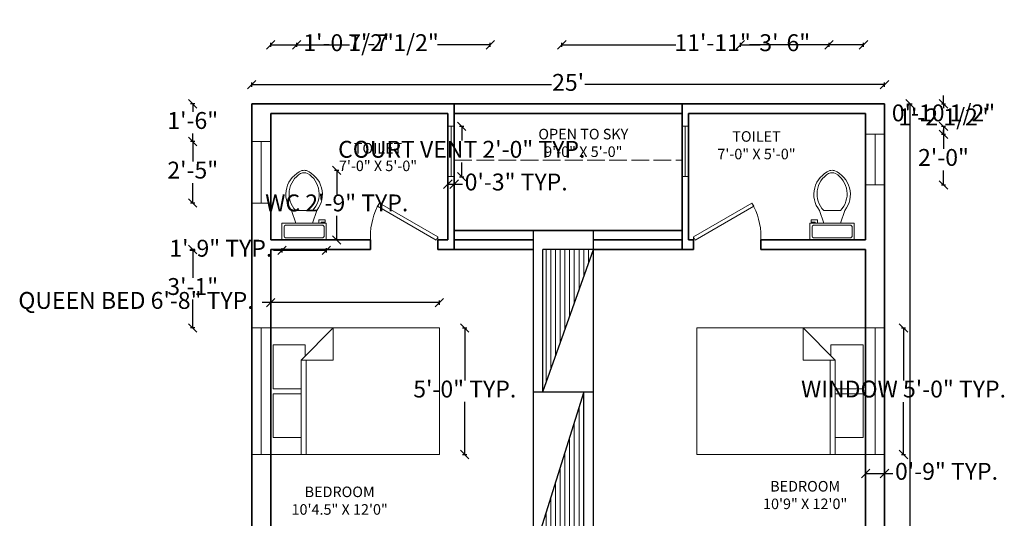
# Model space of a CAD drawing. Units: inches. Extents: x 2558 to 3026, y 433 to 1053.
# Tile 8 of 8: x 2560 to 3026, y 816 to 1053. Entities that reach past the tile are written whole.
import ezdxf

# ---------------------------------------------------------------- set-up
doc = ezdxf.new("R2010")
doc.units = ezdxf.units.IN
doc.linetypes.add('ACAD_ISO02W100', pattern=[15, 12, -3])
for name, color, linetype, lineweight in [('A-ANNO-DIMS', 2, 'Continuous', 18), ('A-AREA-IDEN', 7, 'Continuous', 18), ('A-DOOR', 4, 'Continuous', 18), ('A-FLOR-CASE', 8, 'Continuous', 25), ('A-FLOR-CASE-PATT', 8, 'Continuous', 13), ('A-FLOR-FIXT', 9, 'Continuous', 18), ('A-FLOR-OVHD', 7, 'ACAD_ISO02W100', 18), ('A-FURN', 8, 'Continuous', 18), ('A-GLAZ', 5, 'Continuous', 18), ('A-WALL', 7, 'Continuous', 35)]:
    doc.layers.add(name, color=color, linetype=linetype, lineweight=lineweight)
doc.styles.get("Standard").update_dxf_attribs({"font": 'arial.ttf'})
doc.dimstyles.new('ISO-25', dxfattribs={"dimtxt": 8, "dimasz": 4, "dimexe": 1, "dimexo": 1, "dimgap": 1, "dimtad": 0, "dimtih": 1, "dimtoh": 1, "dimlunit": 3, "dimtxsty": 'Standard', "dimblk": 'OBLIQUE', "dimcen": 2.5, "dimclrt": 1, "dimadec": 0, "dimazin": 0, "dimtfac": 1, "dimtmove": 0, "dimatfit": 3, "dimfxl": 1, "dimfxlon": 1, "dimarcsym": 0})

# ---------------------------------------------------------------- blocks, each defined once
blk = doc.blocks.new('*U6')
for p, q in [((0, 0), (0, -6)), ((-32, 0), (-32, -6))]:
    blk.add_line(p, q)
blk.add_lwpolyline([(0, 0), (-27.71, 16), (-28.59, 14.48), (-0.88, -1.52)], close=True)
blk.add_arc((0, 0), 32, 150, 180)
blk = doc.blocks.new('*U7')
for p, q in [((0, 0), (0, -6)), ((32, 0), (32, -6))]:
    blk.add_line(p, q)
blk.add_lwpolyline([(0, 0), (27.71, 16), (28.59, 14.48), (0.87, -1.52)], close=True)
blk.add_arc((0, 0), 32, 0, 30)
blk = doc.blocks.new('Bed - Queen')
for p, q in [((0, -80.00003), (0, 0)), ((0, 0), (59.99999, 0)), ((59.99999, 0), (59.99999, -80.00003)), ((7.99999, -1.2), (28.79998, -1.2)), ((7.99999, -14.4), (7.99999, -1.2)), ((28.79998, -1.2), (28.79998, -14.4)), ((31.19999, -1.2), (51.99999, -1.2)), ((31.19999, -14.4), (31.19999, -1.2)), ((51.99999, -1.2), (51.99999, -16.4)), ((0, -14.4), (44.8, -14.4)), ((44.8, -16.8), (0, -16.8)), ((59.99999, -29.6), (44.8, -14.4)), ((44.8, -14.4), (44.8, -29.6)), ((51.99999, -16.4), (46.79936, -16.4)), ((44.8, -29.6), (59.99999, -29.6)), ((59.99999, -80.00003), (0, -80.00003))]:
    blk.add_line(p, q)
blk = doc.blocks.new('Toilet - top')
for p, q in [((9.5, -6), (9.5, -2)), ((-10, -8.5), (-8, -8.5)), ((-10, -9.5), (-10, -8.5)), ((-8, -8.5), (-8, -8)), ((-7, -8), (-7, -9.5)), ((-4, -8), (-6, -14)), ((4, -8), (6, -14)), ((-7, -9.5), (-10, -9.5)), ((4, -14), (-4, -14))]:
    blk.add_line(p, q)
blk.add_lwpolyline([(10.5, -8), (10.5, 0), (-10.5, 0), (-10.5, -8)], close=True)
for points in [[(-9.5, -2), (-9.5, -6)], [(8.5, -1), (-8.5, -1)], [(-8.5, -7), (8.5, -7)]]:
    blk.add_lwpolyline(points)
for centre, radius, start, end in [((-8.62, -1.88), 0.884, 81.8699, 188.1301), ((8.62, -1.88), 0.884, 351.8699, 98.1301), ((-8.62, -6.12), 0.884, 171.8699, 278.1301), ((8.62, -6.12), 0.884, 261.8699, 8.1301), ((3.52, -21.58), 12.17, 141.4691, 247.9714), ((4.2, -21.82), 11.33, 136.3677, 238.9468), ((-3.52, -21.58), 12.17, 292.0284, 38.5307), ((-4.2, -21.82), 11.33, 301.053, 43.6321), ((0, -27.88), 4, 245.7318, 294.2682), ((0, -29), 4, 254.8605, 285.1395)]:
    blk.add_arc(centre, radius, start, end)
blk = doc.blocks.new('_Oblique')
at = {"color": 0, "linetype": 'ByBlock', "lineweight": -2}
blk.add_line((-0.5, -0.5), (0.5, 0.5), dxfattribs=at)
blk = doc.blocks.new('*D18')
at = {"layer": 'A-ANNO-DIMS', "color": 0, "lineweight": -2, "transparency": 16777216}
for p, q in [((2669.63, 1020.96), (2669.63, 1022.96)), ((2969.63, 1020.96), (2969.63, 1022.96)), ((2669.63, 1021.96), (2811.78, 1021.96)), ((2969.63, 1021.96), (2827.49, 1021.96))]:
    blk.add_line(p, q, dxfattribs=at)
at = {"layer": 'Defpoints', "color": 0, "transparency": 16777216}
for p in [(2669.63, 1021.96), (2669.63, 1012.82), (2969.63, 1012.82)]:
    blk.add_point(p, dxfattribs=at)
at = {"layer": 'A-ANNO-DIMS', "color": 0, "lineweight": -2, "transparency": 16777216, "xscale": 4, "yscale": 4, "zscale": 4, "rotation": 180}
blk.add_blockref('_Oblique', (2669.63, 1021.96), dxfattribs=at)
at = {"layer": 'A-ANNO-DIMS', "color": 0, "lineweight": -2, "transparency": 16777216, "xscale": 4, "yscale": 4, "zscale": 4}
blk.add_blockref('_Oblique', (2969.63, 1021.96), dxfattribs=at)
at = {"layer": 'A-ANNO-DIMS', "color": 0, "transparency": 16777216, "insert": (2819.63, 1021.96), "char_height": 8, "attachment_point": 5}
blk.add_mtext("25'", dxfattribs=at)
blk = doc.blocks.new('*D19')
at = {"layer": 'A-ANNO-DIMS', "color": 0, "lineweight": -2, "transparency": 16777216}
for p, q in [((2980.65, 1012.82), (2982.65, 1012.82)), ((2981.65, 1012.82), (2981.65, 747.89)), ((2981.65, 472.82), (2981.65, 737.76)), ((2980.65, 472.82), (2982.65, 472.82))]:
    blk.add_line(p, q, dxfattribs=at)
at = {"layer": 'Defpoints', "color": 0, "transparency": 16777216}
for p in [(2969.63, 1012.82), (2969.63, 472.82), (2981.65, 472.82)]:
    blk.add_point(p, dxfattribs=at)
at = {"layer": 'A-ANNO-DIMS', "color": 0, "lineweight": -2, "transparency": 16777216, "xscale": 4, "yscale": 4, "zscale": 4}
for p, rotation in [((2981.65, 1012.82), 90), ((2981.65, 472.82), 270)]:
    blk.add_blockref('_Oblique', p, dxfattribs=dict(at, rotation=rotation))
at = {"layer": 'A-ANNO-DIMS', "color": 0, "transparency": 16777216, "insert": (2981.65, 742.82), "char_height": 8, "attachment_point": 5}
blk.add_mtext("45'", dxfattribs=at)
blk = doc.blocks.new('WIN-COURT-VENT')
for p, q in [((0, 23.85), (3, 23.85)), ((1.5, 23.85), (1.5, 0)), ((0, 0), (3, 0))]:
    blk.add_line(p, q)
blk = doc.blocks.new('WIN-BEDROOM-60IN')
for p, q in [((0, 60), (9, 60)), ((4.5, 60), (4.5, 0)), ((0, 0), (9, 0))]:
    blk.add_line(p, q)
blk = doc.blocks.new('*D23')
at = {"layer": 'A-ANNO-DIMS', "color": 0, "lineweight": -2, "transparency": 16777216}
for p, q in [((2708.95, 981.37), (2710.95, 981.37)), ((2709.95, 981.37), (2709.95, 969.98)), ((2709.95, 948.32), (2709.95, 959.71)), ((2708.95, 948.32), (2710.95, 948.32))]:
    blk.add_line(p, q, dxfattribs=at)
at = {"layer": 'Defpoints', "color": 0, "transparency": 16777216}
for p in [(2704.99, 981.37), (2704.99, 948.32), (2709.95, 948.32)]:
    blk.add_point(p, dxfattribs=at)
at = {"layer": 'A-ANNO-DIMS', "color": 0, "lineweight": -2, "transparency": 16777216, "xscale": 4, "yscale": 4, "zscale": 4}
for p, rotation in [((2709.95, 981.37), 90), ((2709.95, 948.32), 270)]:
    blk.add_blockref('_Oblique', p, dxfattribs=dict(at, rotation=rotation))
at = {"layer": 'A-ANNO-DIMS', "color": 1, "transparency": 16777216, "insert": (2709.95, 964.85), "char_height": 8, "attachment_point": 5}
blk.add_mtext('WC 2\'-9" TYP.', dxfattribs=at)
blk = doc.blocks.new('*D24')
at = {"layer": 'A-ANNO-DIMS', "color": 0, "lineweight": -2, "transparency": 16777216}
for p, q in [((2683.99, 943.37), (2679.99, 943.37)), ((2683.99, 944.37), (2683.99, 942.37)), ((2704.99, 943.37), (2683.99, 943.37)), ((2704.99, 944.37), (2704.99, 942.37))]:
    blk.add_line(p, q, dxfattribs=at)
at = {"layer": 'Defpoints', "color": 0, "transparency": 16777216}
for p in [(2683.99, 948.32), (2704.99, 948.32), (2683.99, 943.37)]:
    blk.add_point(p, dxfattribs=at)
at = {"layer": 'A-ANNO-DIMS', "color": 0, "lineweight": -2, "transparency": 16777216, "xscale": 4, "yscale": 4, "zscale": 4, "rotation": 180}
blk.add_blockref('_Oblique', (2683.99, 943.37), dxfattribs=at)
at = {"layer": 'A-ANNO-DIMS', "color": 0, "lineweight": -2, "transparency": 16777216, "xscale": 4, "yscale": 4, "zscale": 4}
blk.add_blockref('_Oblique', (2704.99, 943.37), dxfattribs=at)
at = {"layer": 'A-ANNO-DIMS', "color": 1, "transparency": 16777216, "insert": (2654.99, 943.37), "char_height": 8, "attachment_point": 5}
blk.add_mtext('1\'-9" TYP.', dxfattribs=at)
blk = doc.blocks.new('*D25')
at = {"layer": 'A-ANNO-DIMS', "color": 0, "lineweight": -2, "transparency": 16777216}
for p, q in [((2678.63, 917.64), (2678.63, 919.64)), ((2758.63, 917.64), (2758.63, 919.64)), ((2678.63, 918.64), (2674.63, 918.64)), ((2758.63, 918.64), (2678.63, 918.64))]:
    blk.add_line(p, q, dxfattribs=at)
at = {"layer": 'Defpoints', "color": 0, "transparency": 16777216}
for p in [(2678.63, 918.64), (2678.63, 906.64), (2758.63, 906.64)]:
    blk.add_point(p, dxfattribs=at)
at = {"layer": 'A-ANNO-DIMS', "color": 0, "lineweight": -2, "transparency": 16777216, "xscale": 4, "yscale": 4, "zscale": 4, "rotation": 180}
blk.add_blockref('_Oblique', (2678.63, 918.64), dxfattribs=at)
at = {"layer": 'A-ANNO-DIMS', "color": 0, "lineweight": -2, "transparency": 16777216, "xscale": 4, "yscale": 4, "zscale": 4}
blk.add_blockref('_Oblique', (2758.63, 918.64), dxfattribs=at)
at = {"layer": 'A-ANNO-DIMS', "color": 1, "transparency": 16777216, "insert": (2614.79, 918.64), "char_height": 8, "attachment_point": 5}
blk.add_mtext('QUEEN BED 6\'-8" TYP.', dxfattribs=at)
blk = doc.blocks.new('*D26')
at = {"layer": 'A-ANNO-DIMS', "color": 0, "lineweight": -2, "transparency": 16777216}
for p, q in [((2769.63, 906.64), (2771.63, 906.64)), ((2770.63, 906.64), (2770.63, 881.73)), ((2770.63, 846.64), (2770.63, 871.56)), ((2769.63, 846.64), (2771.63, 846.64))]:
    blk.add_line(p, q, dxfattribs=at)
at = {"layer": 'Defpoints', "color": 0, "transparency": 16777216}
for p in [(2758.63, 906.64), (2770.63, 906.64), (2758.63, 846.64)]:
    blk.add_point(p, dxfattribs=at)
at = {"layer": 'A-ANNO-DIMS', "color": 0, "lineweight": -2, "transparency": 16777216, "xscale": 4, "yscale": 4, "zscale": 4}
for p, rotation in [((2770.63, 906.64), 90), ((2770.63, 846.64), 270)]:
    blk.add_blockref('_Oblique', p, dxfattribs=dict(at, rotation=rotation))
at = {"layer": 'A-ANNO-DIMS', "color": 1, "transparency": 16777216, "insert": (2770.63, 876.64), "char_height": 8, "attachment_point": 5}
blk.add_mtext('5\'-0" TYP.', dxfattribs=at)
blk = doc.blocks.new('*D35')
at = {"layer": 'A-ANNO-DIMS', "color": 0, "lineweight": -2, "transparency": 16777216}
for p, q in [((2768.21, 1002.18), (2770.21, 1002.18)), ((2769.21, 1002.18), (2769.21, 995.39)), ((2769.21, 978.32), (2769.21, 985.11)), ((2768.21, 978.32), (2770.21, 978.32))]:
    blk.add_line(p, q, dxfattribs=at)
at = {"layer": 'Defpoints', "color": 0, "transparency": 16777216}
for p in [(2765.63, 1002.18), (2769.21, 1002.18), (2765.63, 978.32)]:
    blk.add_point(p, dxfattribs=at)
at = {"layer": 'A-ANNO-DIMS', "color": 0, "lineweight": -2, "transparency": 16777216, "xscale": 4, "yscale": 4, "zscale": 4}
for p, rotation in [((2769.21, 1002.18), 90), ((2769.21, 978.32), 270)]:
    blk.add_blockref('_Oblique', p, dxfattribs=dict(at, rotation=rotation))
at = {"layer": 'A-ANNO-DIMS', "color": 1, "transparency": 16777216, "insert": (2769.21, 990.25), "char_height": 8, "attachment_point": 5}
blk.add_mtext('COURT VENT 2\'-0" TYP.', dxfattribs=at)
blk = doc.blocks.new('*D36')
at = {"layer": 'A-ANNO-DIMS', "color": 0, "lineweight": -2, "transparency": 16777216}
for p, q in [((2762.63, 975.75), (2762.63, 973.75)), ((2765.63, 975.75), (2765.63, 973.75)), ((2762.63, 974.75), (2765.63, 974.75)), ((2765.63, 974.75), (2769.63, 974.75))]:
    blk.add_line(p, q, dxfattribs=at)
at = {"layer": 'Defpoints', "color": 0, "transparency": 16777216}
for p in [(2762.63, 978.32), (2765.63, 978.32), (2765.63, 974.75)]:
    blk.add_point(p, dxfattribs=at)
at = {"layer": 'A-ANNO-DIMS', "color": 0, "lineweight": -2, "transparency": 16777216, "xscale": 4, "yscale": 4, "zscale": 4, "rotation": 180}
blk.add_blockref('_Oblique', (2762.63, 974.75), dxfattribs=at)
at = {"layer": 'A-ANNO-DIMS', "color": 0, "lineweight": -2, "transparency": 16777216, "xscale": 4, "yscale": 4, "zscale": 4}
blk.add_blockref('_Oblique', (2765.63, 974.75), dxfattribs=at)
at = {"layer": 'A-ANNO-DIMS', "color": 1, "transparency": 16777216, "insert": (2795.01, 974.75), "char_height": 8, "attachment_point": 5}
blk.add_mtext('0\'-3" TYP.', dxfattribs=at)
blk = doc.blocks.new('*D37')
at = {"layer": 'A-ANNO-DIMS', "color": 0, "lineweight": -2, "transparency": 16777216}
for p, q in [((2977.63, 906.64), (2979.63, 906.64)), ((2978.63, 906.64), (2978.63, 881.78)), ((2978.63, 846.64), (2978.63, 871.5)), ((2977.63, 846.64), (2979.63, 846.64))]:
    blk.add_line(p, q, dxfattribs=at)
at = {"layer": 'Defpoints', "color": 0, "transparency": 16777216}
for p in [(2969.63, 906.64), (2978.63, 906.64), (2969.63, 846.64)]:
    blk.add_point(p, dxfattribs=at)
at = {"layer": 'A-ANNO-DIMS', "color": 0, "lineweight": -2, "transparency": 16777216, "xscale": 4, "yscale": 4, "zscale": 4}
for p, rotation in [((2978.63, 906.64), 90), ((2978.63, 846.64), 270)]:
    blk.add_blockref('_Oblique', p, dxfattribs=dict(at, rotation=rotation))
at = {"layer": 'A-ANNO-DIMS', "color": 1, "transparency": 16777216, "insert": (2978.63, 876.64), "char_height": 8, "attachment_point": 5}
blk.add_mtext('WINDOW 5\'-0" TYP.', dxfattribs=at)
blk = doc.blocks.new('*D38')
at = {"layer": 'A-ANNO-DIMS', "color": 0, "lineweight": -2, "transparency": 16777216}
for p, q in [((2960.63, 838.64), (2960.63, 836.64)), ((2960.63, 837.64), (2969.63, 837.64)), ((2969.63, 838.64), (2969.63, 836.64)), ((2969.63, 837.64), (2973.63, 837.64))]:
    blk.add_line(p, q, dxfattribs=at)
at = {"layer": 'Defpoints', "color": 0, "transparency": 16777216}
for p in [(2960.63, 846.64), (2969.63, 846.64), (2969.63, 837.64)]:
    blk.add_point(p, dxfattribs=at)
at = {"layer": 'A-ANNO-DIMS', "color": 0, "lineweight": -2, "transparency": 16777216, "xscale": 4, "yscale": 4, "zscale": 4, "rotation": 180}
blk.add_blockref('_Oblique', (2960.63, 837.64), dxfattribs=at)
at = {"layer": 'A-ANNO-DIMS', "color": 0, "lineweight": -2, "transparency": 16777216, "xscale": 4, "yscale": 4, "zscale": 4}
blk.add_blockref('_Oblique', (2969.63, 837.64), dxfattribs=at)
at = {"layer": 'A-ANNO-DIMS', "color": 1, "transparency": 16777216, "insert": (2999.01, 837.64), "char_height": 8, "attachment_point": 5}
blk.add_mtext('0\'-9" TYP.', dxfattribs=at)
blk = doc.blocks.new('*D48')
at = {"layer": 'A-ANNO-DIMS', "color": 0, "lineweight": -2, "transparency": 16777216}
for p, q in [((2725.89, 445.87), (2725.89, 443.87)), ((2725.89, 444.87), (2730.19, 444.87)), ((2757.89, 444.87), (2753.59, 444.87)), ((2757.89, 445.87), (2757.89, 443.87))]:
    blk.add_line(p, q, dxfattribs=at)
at = {"layer": 'Defpoints', "color": 0, "transparency": 16777216}
for p in [(2725.89, 943.82), (2757.89, 943.82), (2757.89, 444.87)]:
    blk.add_point(p, dxfattribs=at)
at = {"layer": 'A-ANNO-DIMS', "color": 0, "lineweight": -2, "transparency": 16777216, "xscale": 4, "yscale": 4, "zscale": 4, "rotation": 180}
blk.add_blockref('_Oblique', (2725.89, 444.87), dxfattribs=at)
at = {"layer": 'A-ANNO-DIMS', "color": 0, "lineweight": -2, "transparency": 16777216, "xscale": 4, "yscale": 4, "zscale": 4}
blk.add_blockref('_Oblique', (2757.89, 444.87), dxfattribs=at)
at = {"layer": 'A-ANNO-DIMS', "color": 1, "transparency": 16777216, "insert": (2741.89, 444.87), "char_height": 8, "attachment_point": 5}
blk.add_mtext('2\'-8"', dxfattribs=at)
blk = doc.blocks.new('*D52')
at = {"layer": 'A-ANNO-DIMS', "color": 0, "lineweight": -2, "transparency": 16777216}
for p, q in [((2642.68, 994.97), (2640.68, 994.97)), ((2641.68, 994.97), (2641.68, 985.47)), ((2641.68, 965.81), (2641.68, 975.3)), ((2642.68, 965.81), (2640.68, 965.81))]:
    blk.add_line(p, q, dxfattribs=at)
at = {"layer": 'Defpoints', "color": 0, "transparency": 16777216}
for p in [(2641.68, 994.97), (2669.63, 994.97), (2669.63, 965.81)]:
    blk.add_point(p, dxfattribs=at)
at = {"layer": 'A-ANNO-DIMS', "color": 0, "lineweight": -2, "transparency": 16777216, "xscale": 4, "yscale": 4, "zscale": 4}
for p, rotation in [((2641.68, 994.97), 90), ((2641.68, 965.81), 270)]:
    blk.add_blockref('_Oblique', p, dxfattribs=dict(at, rotation=rotation))
at = {"layer": 'A-ANNO-DIMS', "color": 1, "transparency": 16777216, "insert": (2641.68, 980.39), "char_height": 8, "attachment_point": 5}
blk.add_mtext('2\'-5"', dxfattribs=at)
blk = doc.blocks.new('*D53')
at = {"layer": 'A-ANNO-DIMS', "color": 0, "lineweight": -2, "transparency": 16777216}
for p, q in [((2996.58, 998.39), (2998.58, 998.39)), ((2997.58, 998.39), (2997.58, 991.47)), ((2997.58, 974.39), (2997.58, 981.31)), ((2996.58, 974.39), (2998.58, 974.39))]:
    blk.add_line(p, q, dxfattribs=at)
at = {"layer": 'Defpoints', "color": 0, "transparency": 16777216}
for p in [(2969.63, 998.39), (2997.58, 998.39), (2969.63, 974.39)]:
    blk.add_point(p, dxfattribs=at)
at = {"layer": 'A-ANNO-DIMS', "color": 0, "lineweight": -2, "transparency": 16777216, "xscale": 4, "yscale": 4, "zscale": 4}
for p, rotation in [((2997.58, 998.39), 90), ((2997.58, 974.39), 270)]:
    blk.add_blockref('_Oblique', p, dxfattribs=dict(at, rotation=rotation))
at = {"layer": 'A-ANNO-DIMS', "color": 1, "transparency": 16777216, "insert": (2997.58, 986.39), "char_height": 8, "attachment_point": 5}
blk.add_mtext('2\'-0"', dxfattribs=at)
blk = doc.blocks.new('*D58')
at = {"layer": 'A-ANNO-DIMS', "color": 0, "lineweight": -2, "transparency": 16777216}
for p, q in [((2901.29, 1039.77), (2901.29, 1041.77)), ((2943.34, 1039.77), (2943.34, 1041.77)), ((2901.29, 1040.77), (2910.69, 1040.77)), ((2943.34, 1040.77), (2933.95, 1040.77))]:
    blk.add_line(p, q, dxfattribs=at)
at = {"layer": 'Defpoints', "color": 0, "transparency": 16777216}
for p in [(2943.34, 1040.77), (2901.29, 649.82), (2943.34, 649.82)]:
    blk.add_point(p, dxfattribs=at)
at = {"layer": 'A-ANNO-DIMS', "color": 0, "lineweight": -2, "transparency": 16777216, "xscale": 4, "yscale": 4, "zscale": 4, "rotation": 180}
blk.add_blockref('_Oblique', (2901.29, 1040.77), dxfattribs=at)
at = {"layer": 'A-ANNO-DIMS', "color": 0, "lineweight": -2, "transparency": 16777216, "xscale": 4, "yscale": 4, "zscale": 4}
blk.add_blockref('_Oblique', (2943.34, 1040.77), dxfattribs=at)
at = {"layer": 'A-ANNO-DIMS', "color": 1, "transparency": 16777216, "insert": (2922.32, 1040.77), "char_height": 8, "attachment_point": 5}
blk.add_mtext('3\'-6"', dxfattribs=at)
blk = doc.blocks.new('*D59')
at = {"layer": 'A-ANNO-DIMS', "color": 0, "lineweight": -2, "transparency": 16777216}
for p, q in [((2690.99, 1039.77), (2690.99, 1041.77)), ((2782.72, 1039.77), (2782.72, 1041.77)), ((2690.99, 1040.77), (2715.93, 1040.77)), ((2782.72, 1040.77), (2757.77, 1040.77))]:
    blk.add_line(p, q, dxfattribs=at)
at = {"layer": 'Defpoints', "color": 0, "transparency": 16777216}
for p in [(2782.72, 1040.77), (2690.99, 658.82), (2782.72, 658.82)]:
    blk.add_point(p, dxfattribs=at)
at = {"layer": 'A-ANNO-DIMS', "color": 0, "lineweight": -2, "transparency": 16777216, "xscale": 4, "yscale": 4, "zscale": 4, "rotation": 180}
blk.add_blockref('_Oblique', (2690.99, 1040.77), dxfattribs=at)
at = {"layer": 'A-ANNO-DIMS', "color": 0, "lineweight": -2, "transparency": 16777216, "xscale": 4, "yscale": 4, "zscale": 4}
blk.add_blockref('_Oblique', (2782.72, 1040.77), dxfattribs=at)
at = {"layer": 'A-ANNO-DIMS', "color": 1, "transparency": 16777216, "insert": (2736.85, 1040.77), "char_height": 8, "attachment_point": 5}
blk.add_mtext('7\'-7 1/2"', dxfattribs=at)
blk = doc.blocks.new('*D61')
at = {"layer": 'A-ANNO-DIMS', "color": 0, "lineweight": -2, "transparency": 16777216}
for p, q in [((2642.68, 1012.82), (2640.68, 1012.82)), ((2641.68, 1012.82), (2641.68, 1008.98)), ((2642.68, 994.97), (2640.68, 994.97)), ((2641.68, 994.97), (2641.68, 998.81))]:
    blk.add_line(p, q, dxfattribs=at)
at = {"layer": 'Defpoints', "color": 0, "transparency": 16777216}
for p in [(2641.68, 1012.82), (2669.63, 1012.82), (2669.63, 994.97)]:
    blk.add_point(p, dxfattribs=at)
at = {"layer": 'A-ANNO-DIMS', "color": 0, "lineweight": -2, "transparency": 16777216, "xscale": 4, "yscale": 4, "zscale": 4}
for p, rotation in [((2641.68, 1012.82), 90), ((2641.68, 994.97), 270)]:
    blk.add_blockref('_Oblique', p, dxfattribs=dict(at, rotation=rotation))
at = {"layer": 'A-ANNO-DIMS', "color": 1, "transparency": 16777216, "insert": (2641.68, 1003.9), "char_height": 8, "attachment_point": 5}
blk.add_mtext('1\'-6"', dxfattribs=at)
blk = doc.blocks.new('*D62')
at = {"layer": 'A-ANNO-DIMS', "color": 0, "lineweight": -2, "transparency": 16777216}
for p, q in [((2997.58, 1012.82), (2997.58, 1016.82)), ((2996.58, 1012.82), (2998.58, 1012.82)), ((2997.58, 1012.82), (2997.58, 1012.64)), ((2996.58, 1002.18), (2998.58, 1002.18)), ((2997.58, 1002.18), (2997.58, 1002.36)), ((2997.58, 1002.18), (2997.58, 998.18))]:
    blk.add_line(p, q, dxfattribs=at)
at = {"layer": 'Defpoints', "color": 0, "transparency": 16777216}
for p in [(2765.63, 1012.82), (2997.58, 1012.82), (2765.63, 1002.18)]:
    blk.add_point(p, dxfattribs=at)
at = {"layer": 'A-ANNO-DIMS', "color": 0, "lineweight": -2, "transparency": 16777216, "xscale": 4, "yscale": 4, "zscale": 4}
for p, rotation in [((2997.58, 1012.82), 270), ((2997.58, 1002.18), 90)]:
    blk.add_blockref('_Oblique', p, dxfattribs=dict(at, rotation=rotation))
at = {"layer": 'A-ANNO-DIMS', "color": 1, "transparency": 16777216, "insert": (2997.58, 1007.5), "char_height": 8, "attachment_point": 5}
blk.add_mtext('0\'-10 1/2"', dxfattribs=at)
blk = doc.blocks.new('*D63')
at = {"layer": 'A-ANNO-DIMS', "color": 0, "lineweight": -2, "transparency": 16777216}
for p, q in [((2757.89, 445.87), (2757.89, 443.87)), ((2757.89, 444.87), (2765.63, 444.87)), ((2765.63, 445.87), (2765.63, 443.87)), ((2765.63, 444.87), (2769.63, 444.87))]:
    blk.add_line(p, q, dxfattribs=at)
at = {"layer": 'Defpoints', "color": 0, "transparency": 16777216}
for p in [(2757.89, 943.82), (2765.63, 943.82), (2765.63, 444.87)]:
    blk.add_point(p, dxfattribs=at)
at = {"layer": 'A-ANNO-DIMS', "color": 0, "lineweight": -2, "transparency": 16777216, "xscale": 4, "yscale": 4, "zscale": 4, "rotation": 180}
blk.add_blockref('_Oblique', (2757.89, 444.87), dxfattribs=at)
at = {"layer": 'A-ANNO-DIMS', "color": 0, "lineweight": -2, "transparency": 16777216, "xscale": 4, "yscale": 4, "zscale": 4}
blk.add_blockref('_Oblique', (2765.63, 444.87), dxfattribs=at)
at = {"layer": 'A-ANNO-DIMS', "color": 1, "transparency": 16777216, "insert": (2790.59, 444.87), "char_height": 8, "attachment_point": 5}
blk.add_mtext('0\'-7 1/2"', dxfattribs=at)
blk = doc.blocks.new('*D64')
at = {"layer": 'A-ANNO-DIMS', "color": 0, "lineweight": -2, "transparency": 16777216}
for p, q in [((2996.58, 1012.82), (2998.58, 1012.82)), ((2997.58, 1012.82), (2997.58, 1010.74)), ((2997.58, 998.39), (2997.58, 1000.47)), ((2996.58, 998.39), (2998.58, 998.39))]:
    blk.add_line(p, q, dxfattribs=at)
at = {"layer": 'Defpoints', "color": 0, "transparency": 16777216}
for p in [(2969.63, 1012.82), (2997.58, 1012.82), (2969.63, 998.39)]:
    blk.add_point(p, dxfattribs=at)
at = {"layer": 'A-ANNO-DIMS', "color": 0, "lineweight": -2, "transparency": 16777216, "xscale": 4, "yscale": 4, "zscale": 4}
for p, rotation in [((2997.58, 1012.82), 90), ((2997.58, 998.39), 270)]:
    blk.add_blockref('_Oblique', p, dxfattribs=dict(at, rotation=rotation))
at = {"layer": 'A-ANNO-DIMS', "color": 1, "transparency": 16777216, "insert": (2997.58, 1005.61), "char_height": 8, "attachment_point": 5}
blk.add_mtext('1\'-2 1/2"', dxfattribs=at)
blk = doc.blocks.new('*D65')
at = {"layer": 'A-ANNO-DIMS', "color": 0, "lineweight": -2, "transparency": 16777216}
for p, q in [((2642.68, 943.82), (2640.68, 943.82)), ((2641.68, 943.82), (2641.68, 930.32)), ((2641.68, 906.64), (2641.68, 920.15)), ((2642.68, 906.64), (2640.68, 906.64))]:
    blk.add_line(p, q, dxfattribs=at)
at = {"layer": 'Defpoints', "color": 0, "transparency": 16777216}
for p in [(2641.68, 943.82), (2678.63, 943.82), (2678.63, 906.64)]:
    blk.add_point(p, dxfattribs=at)
at = {"layer": 'A-ANNO-DIMS', "color": 0, "lineweight": -2, "transparency": 16777216, "xscale": 4, "yscale": 4, "zscale": 4}
for p, rotation in [((2641.68, 943.82), 90), ((2641.68, 906.64), 270)]:
    blk.add_blockref('_Oblique', p, dxfattribs=dict(at, rotation=rotation))
at = {"layer": 'A-ANNO-DIMS', "color": 1, "transparency": 16777216, "insert": (2641.68, 925.23), "char_height": 8, "attachment_point": 5}
blk.add_mtext('3\'-1"', dxfattribs=at)
blk = doc.blocks.new('*D70')
at = {"layer": 'A-ANNO-DIMS', "color": 0, "lineweight": -2, "transparency": 16777216}
for p, q in [((2678.63, 1039.77), (2678.63, 1041.77)), ((2690.99, 1039.77), (2690.99, 1041.77)), ((2678.63, 1040.77), (2690.99, 1040.77)), ((2690.99, 1040.77), (2694.99, 1040.77))]:
    blk.add_line(p, q, dxfattribs=at)
at = {"layer": 'Defpoints', "color": 0, "transparency": 16777216}
for p in [(2690.99, 1040.77), (2678.63, 658.82), (2690.99, 658.82)]:
    blk.add_point(p, dxfattribs=at)
at = {"layer": 'A-ANNO-DIMS', "color": 0, "lineweight": -2, "transparency": 16777216, "xscale": 4, "yscale": 4, "zscale": 4, "rotation": 180}
blk.add_blockref('_Oblique', (2678.63, 1040.77), dxfattribs=at)
at = {"layer": 'A-ANNO-DIMS', "color": 0, "lineweight": -2, "transparency": 16777216, "xscale": 4, "yscale": 4, "zscale": 4}
blk.add_blockref('_Oblique', (2690.99, 1040.77), dxfattribs=at)
at = {"layer": 'A-ANNO-DIMS', "color": 1, "transparency": 16777216, "insert": (2715.56, 1040.77), "char_height": 8, "attachment_point": 5}
blk.add_mtext('1\'-0 1/2"', dxfattribs=at)
blk = doc.blocks.new('*D73')
at = {"layer": 'A-ANNO-DIMS', "color": 0, "lineweight": -2, "transparency": 16777216}
for p, q in [((2816.63, 1039.77), (2816.63, 1041.77)), ((2959.63, 1039.77), (2959.63, 1041.77)), ((2816.63, 1040.77), (2870.66, 1040.77)), ((2959.63, 1040.77), (2905.6, 1040.77))]:
    blk.add_line(p, q, dxfattribs=at)
at = {"layer": 'Defpoints', "color": 0, "transparency": 16777216}
for p in [(2959.63, 1040.77), (2816.63, 481.83), (2959.63, 481.82)]:
    blk.add_point(p, dxfattribs=at)
at = {"layer": 'A-ANNO-DIMS', "color": 0, "lineweight": -2, "transparency": 16777216, "xscale": 4, "yscale": 4, "zscale": 4, "rotation": 180}
blk.add_blockref('_Oblique', (2816.63, 1040.77), dxfattribs=at)
at = {"layer": 'A-ANNO-DIMS', "color": 0, "lineweight": -2, "transparency": 16777216, "xscale": 4, "yscale": 4, "zscale": 4}
blk.add_blockref('_Oblique', (2959.63, 1040.77), dxfattribs=at)
at = {"layer": 'A-ANNO-DIMS', "color": 1, "transparency": 16777216, "insert": (2888.13, 1040.77), "char_height": 8, "attachment_point": 5}
blk.add_mtext('11\'-11"', dxfattribs=at)
blk = doc.blocks.new('*D76')
at = {"layer": 'A-ANNO-DIMS', "color": 0, "lineweight": -2, "transparency": 16777216}
for p, q in [((2879.03, 445.87), (2879.03, 443.87)), ((2879.03, 444.87), (2883.32, 444.87)), ((2911.03, 444.87), (2906.73, 444.87)), ((2911.03, 445.87), (2911.03, 443.87))]:
    blk.add_line(p, q, dxfattribs=at)
at = {"layer": 'Defpoints', "color": 0, "transparency": 16777216}
for p in [(2879.03, 943.82), (2911.03, 943.82), (2911.03, 444.87)]:
    blk.add_point(p, dxfattribs=at)
at = {"layer": 'A-ANNO-DIMS', "color": 0, "lineweight": -2, "transparency": 16777216, "xscale": 4, "yscale": 4, "zscale": 4, "rotation": 180}
blk.add_blockref('_Oblique', (2879.03, 444.87), dxfattribs=at)
at = {"layer": 'A-ANNO-DIMS', "color": 0, "lineweight": -2, "transparency": 16777216, "xscale": 4, "yscale": 4, "zscale": 4}
blk.add_blockref('_Oblique', (2911.03, 444.87), dxfattribs=at)
at = {"layer": 'A-ANNO-DIMS', "color": 1, "transparency": 16777216, "insert": (2895.03, 444.87), "char_height": 8, "attachment_point": 5}
blk.add_mtext('2\'-8"', dxfattribs=at)

msp = doc.modelspace()

# ---------------------------------------------------------------- hatches: boundary and pattern name
at = {"layer": 'A-FLOR-CASE-PATT'}
h = msp.add_hatch(dxfattribs=at)
h.set_pattern_fill('ANSI31', color=256, scale=0.7, angle=45)
h.set_pattern_definition([(90, (0, 4.5), (-2.2225, 0), [])])
h.paths.add_polyline_path([(2831.633, 943.825), (2807.633, 943.825), (2807.633, 876.325)])
h.paths.add_polyline_path([(2827.133, 876.325), (2803.133, 799.825), (2827.133, 799.825)])

# ---------------------------------------------------------------- linework, layer by layer
at = {"layer": 'A-FLOR-CASE'}
for p, q in [((2803.133, 952.825), (2803.133, 799.825)), ((2831.633, 799.825), (2831.633, 952.825)), ((2807.633, 876.325), (2807.633, 943.825)), ((2807.633, 876.325), (2831.633, 943.825)), ((2831.633, 943.825), (2807.633, 943.825)), ((2803.133, 876.325), (2831.633, 876.325)), ((2803.133, 876.325), (2807.633, 876.325)), ((2827.133, 876.325), (2803.133, 799.825)), ((2827.133, 799.825), (2827.133, 876.325))]:
    msp.add_line(p, q, dxfattribs=at)
at = {"layer": 'A-FLOR-OVHD', "ltscale": 0.7}
msp.add_line((2765.633, 986.197), (2873.633, 986.197), dxfattribs=at)
at = {"layer": 'A-GLAZ'}
for p, q in [((2678.633, 994.966), (2669.633, 994.966)), ((2674.133, 994.966), (2674.133, 965.808)), ((2960.633, 998.39), (2969.633, 998.39)), ((2965.133, 998.39), (2965.133, 974.39)), ((2960.633, 974.39), (2969.633, 974.39)), ((2678.633, 965.808), (2669.633, 965.808))]:
    msp.add_line(p, q, dxfattribs=at)
at = {"layer": 'A-WALL'}
for p, q in [((2669.633, 1012.825), (2669.633, 472.825)), ((2765.633, 1012.825), (2669.633, 1012.825)), ((2678.633, 1008.325), (2678.633, 948.325)), ((2762.633, 1008.325), (2678.633, 1008.325)), ((2762.633, 1008.325), (2762.633, 948.325)), ((2765.633, 1012.825), (2765.633, 943.825)), ((2765.633, 1012.825), (2873.633, 1012.825)), ((2873.633, 1008.325), (2765.633, 1008.325)), ((2969.633, 1012.825), (2873.633, 1012.825)), ((2873.633, 943.825), (2873.633, 1012.825)), ((2960.633, 1008.325), (2876.633, 1008.325)), ((2876.633, 948.325), (2876.633, 1008.325)), ((2960.633, 948.325), (2960.633, 1008.325)), ((2969.633, 472.825), (2969.633, 1012.825)), ((2803.133, 952.825), (2765.633, 952.825)), ((2831.633, 952.825), (2803.133, 952.825)), ((2873.633, 952.825), (2831.633, 952.825)), ((2725.892, 948.325), (2678.633, 948.325)), ((2725.892, 948.325), (2725.892, 943.825)), ((2762.633, 948.325), (2757.892, 948.325)), ((2757.892, 948.325), (2757.892, 943.825)), ((2803.133, 948.325), (2765.633, 948.325)), ((2873.633, 948.325), (2831.633, 948.325)), ((2879.025, 948.325), (2876.633, 948.325)), ((2879.025, 948.325), (2879.025, 943.825)), ((2960.633, 948.325), (2911.025, 948.325)), ((2911.025, 948.325), (2911.025, 943.825)), ((2678.633, 943.825), (2678.633, 799.825)), ((2725.892, 943.825), (2678.633, 943.825)), ((2765.633, 943.825), (2757.892, 943.825)), ((2803.133, 943.825), (2765.633, 943.825)), ((2873.633, 943.825), (2831.633, 943.825)), ((2879.025, 943.825), (2873.633, 943.825)), ((2960.633, 943.825), (2911.025, 943.825)), ((2960.633, 799.825), (2960.633, 943.825))]:
    msp.add_line(p, q, dxfattribs=at)

# ---------------------------------------------------------------- block references
at = {"layer": 'A-DOOR'}
for name, p in [('*U6', (2757.892, 949.825)), ('*U7', (2879.025, 949.825))]:
    msp.add_blockref(name, p, dxfattribs=at)
at = {"layer": 'A-FLOR-FIXT', "rotation": 180}
msp.add_blockref('Toilet - top', (2694.491, 948.325), dxfattribs=at)
at = {"layer": 'A-FLOR-FIXT', "xscale": -1, "rotation": 180}
msp.add_blockref('Toilet - top', (2944.774, 948.325), dxfattribs=at)
at = {"layer": 'A-FURN', "rotation": 90}
msp.add_blockref('Bed - Queen', (2678.633, 846.642), dxfattribs=at)
at = {"layer": 'A-FURN', "xscale": -1, "rotation": 270}
msp.add_blockref('Bed - Queen', (2960.633, 846.642), dxfattribs=at)
at = {"layer": 'A-GLAZ'}
for name, p in [('WIN-COURT-VENT', (2762.633, 978.325)), ('WIN-COURT-VENT', (2873.633, 978.325)), ('WIN-BEDROOM-60IN', (2960.633, 846.642))]:
    msp.add_blockref(name, p, dxfattribs=at)
at = {"layer": 'A-GLAZ', "rotation": 180}
msp.add_blockref('WIN-BEDROOM-60IN', (2678.632, 906.641), dxfattribs=at)

# ---------------------------------------------------------------- texts
at = {"layer": 'A-AREA-IDEN', "char_height": 5, "attachment_point": 1}
for s, width, insert in [('\\pxqc;OPEN TO SKY\\P9\'-0" X 5\'-0"', 60.80407, (2796.439, 1000.993)), ('\\pxqc;TOILET\\P7\'-0" X 5\'-0"', 39.67927, (2889.084, 999.88)), ('\\pxqc;TOILET\\P7\'-0" X 5\'-0"', 46.06135, (2706.481, 994.281)), ('\\pxqc;BEDROOM\\P10\'4.5" X 12\'0"', 46.06135, (2688.304, 831.457)), ('\\pxqc;BEDROOM\\P10\'9" X 12\'0"', 46.06135, (2908.969, 834.113))]:
    msp.add_mtext_dynamic_manual_height_columns(s, width=width, gutter_width=12.5, heights=[0], dxfattribs=dict(at, insert=insert))

# ---------------------------------------------------------------- dimensions: what is measured, and where the dimension line sits
at = {"layer": 'A-ANNO-DIMS'}
for base, p1, p2, picture, middle in [((2690.987, 1040.775), (2678.633, 658.825), (2690.987, 658.825), '*D70', (2715.564, 1040.775)), ((2782.721, 1040.775), (2690.987, 658.825), (2782.721, 658.825), '*D59', (2736.854, 1040.775)), ((2959.633, 1040.775), (2816.633, 481.827), (2959.633, 481.825), '*D73', (2888.133, 1040.775)), ((2943.3439, 1040.7746), (2901.2944, 649.8246), (2943.3439, 649.8246), '*D58', (2922.3191, 1040.7746)), ((2757.892, 444.875), (2725.892, 943.825), (2757.892, 943.825), '*D48', (2741.892, 444.875)), ((2765.633, 444.875), (2757.892, 943.825), (2765.633, 943.825), '*D63', (2790.586, 444.875)), ((2911.025, 444.875), (2879.025, 943.825), (2911.025, 943.825), '*D76', (2895.025, 444.875))]:
    dim = msp.add_linear_dim(base=base, p1=p1, p2=p2, dimstyle='ISO-25', override={"dimdec": 1, "dimlfac": 1, "dimrnd": 0, "dimzin": 1, "dimdsep": 46, "dimlunit": 4, "dimfrac": 2}, dxfattribs=at)
    dim.commit()
    dim.dimension.update_dxf_attribs({"geometry": picture, "text_midpoint": middle})
dim = msp.add_linear_dim(base=(2669.633, 1021.956), p1=(2969.633, 1012.825), p2=(2669.633, 1012.825), dimstyle='ISO-25', override={"dimclrd": 0, "dimclre": 0, "dimclrt": 0}, dxfattribs=at)
dim.commit()
dim.dimension.update_dxf_attribs({"geometry": '*D18', "text_midpoint": (2819.633, 1021.956), "dimtype": 160})
for base, p1, p2, override, picture, middle in [((2997.583, 1012.825), (2765.633, 1002.176), (2765.633, 1012.825), {"dimdec": 1, "dimlfac": 1, "dimrnd": 0, "dimzin": 1, "dimdsep": 46, "dimlunit": 4, "dimfrac": 2}, '*D62', (2997.583, 1007.501)), ((2997.583, 1012.825), (2969.633, 998.39), (2969.633, 1012.825), {"dimdec": 1, "dimlfac": 1, "dimrnd": 0, "dimzin": 1, "dimdsep": 46, "dimlunit": 4, "dimfrac": 2}, '*D64', (2997.583, 1005.607)), ((2641.683, 1012.825), (2669.633, 994.966), (2669.633, 1012.825), {"dimdec": 1, "dimlfac": 1, "dimrnd": 0, "dimzin": 1, "dimdsep": 46, "dimlunit": 4, "dimfrac": 2}, '*D61', (2641.683, 1003.895)), ((2981.646, 472.825), (2969.633, 1012.825), (2969.633, 472.825), {"dimclrd": 0, "dimclre": 0, "dimclrt": 0}, '*D19', (2981.646, 742.825)), ((2997.583, 998.39), (2969.633, 974.39), (2969.633, 998.39), {"dimdec": 1, "dimlfac": 1, "dimrnd": 0, "dimzin": 1, "dimdsep": 46, "dimlunit": 4, "dimfrac": 2}, '*D53', (2997.583, 986.39)), ((2641.683, 994.966), (2669.633, 965.808), (2669.633, 994.966), {"dimdec": 1, "dimlfac": 1, "dimrnd": 0, "dimzin": 1, "dimdsep": 46, "dimlunit": 4, "dimfrac": 2}, '*D52', (2641.683, 980.387)), ((2641.683, 943.825), (2678.633, 906.642), (2678.633, 943.825), {"dimdec": 1, "dimlfac": 1, "dimrnd": 0, "dimzin": 1, "dimdsep": 46, "dimlunit": 4, "dimfrac": 2}, '*D65', (2641.683, 925.233))]:
    dim = msp.add_linear_dim(base=base, p1=p1, p2=p2, angle=90, dimstyle='ISO-25', override=override, dxfattribs=at)
    dim.commit()
    dim.dimension.update_dxf_attribs({"geometry": picture, "text_midpoint": middle})
for base, p1, p2, angle, text, picture, middle in [((2769.21, 1002.176), (2765.633, 978.325), (2765.633, 1002.176), 90, 'COURT VENT <> TYP.', '*D35', (2769.21, 990.251)), ((2709.948, 948.325), (2704.991, 981.371), (2704.991, 948.325), 270, 'WC <> TYP.', '*D23', (2709.948, 964.848)), ((2683.991, 943.368), (2704.991, 948.325), (2683.991, 948.325), 180, '<> TYP.', '*D24', (2654.986, 943.368)), ((2678.633, 918.642), (2758.633, 906.642), (2678.633, 906.642), 180, 'QUEEN BED <> TYP.', '*D25', (2614.792, 918.642)), ((2770.633, 906.642), (2758.633, 846.642), (2758.633, 906.642), 90, '<> TYP.', '*D26', (2770.633, 876.642)), ((2978.633, 906.642), (2969.633, 846.642), (2969.633, 906.642), 90, 'WINDOW <> TYP.', '*D37', (2978.633, 876.642))]:
    dim = msp.add_linear_dim(base=base, p1=p1, p2=p2, angle=angle, text=text, dimstyle='ISO-25', override={"dimdec": 1, "dimlfac": 1, "dimrnd": 0, "dimzin": 1, "dimdsep": 46, "dimlunit": 4, "dimfrac": 2}, dxfattribs=at)
    dim.commit()
    dim.dimension.update_dxf_attribs({"geometry": picture, "text_midpoint": middle})
for base, p1, p2, picture, middle in [((2765.633, 974.747), (2762.633, 978.325), (2765.633, 978.325), '*D36', (2795.015, 974.747)), ((2969.633, 837.642), (2960.633, 846.642), (2969.633, 846.642), '*D38', (2999.015, 837.642))]:
    dim = msp.add_linear_dim(base=base, p1=p1, p2=p2, text='<> TYP.', dimstyle='ISO-25', override={"dimdec": 1, "dimlfac": 1, "dimrnd": 0, "dimzin": 1, "dimdsep": 46, "dimlunit": 4, "dimfrac": 2}, dxfattribs=at)
    dim.commit()
    dim.dimension.update_dxf_attribs({"geometry": picture, "text_midpoint": middle})

doc.saveas('drawing.dxf')
